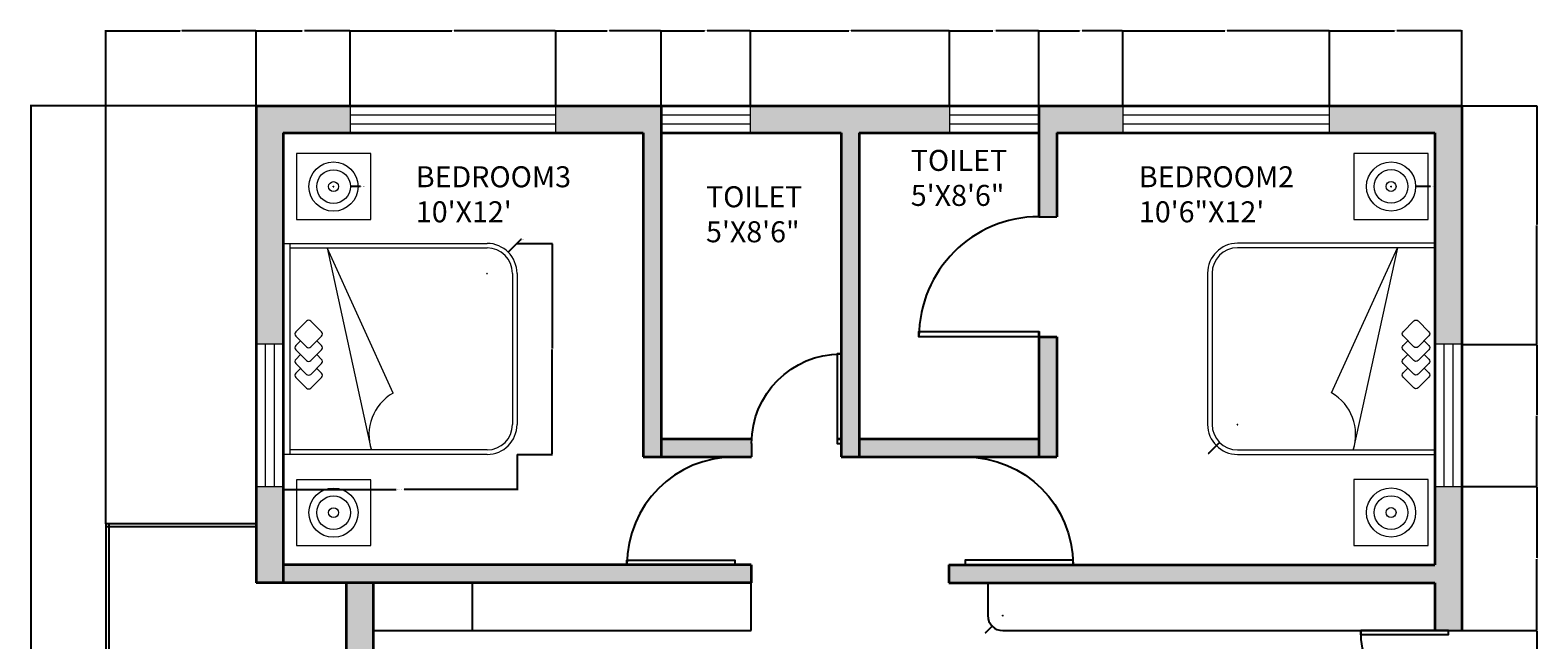
# Model space of a CAD drawing. Units: inches. Extents: x 2764 to 3282, y 1588 to 2106.
# Tile 2 of 2: x 2764 to 3267, y 1903 to 2106. Entities that reach past the tile are written whole.
import ezdxf

# ---------------------------------------------------------------- set-up
doc = ezdxf.new("R2010")
doc.units = ezdxf.units.IN
for name, color, linetype, lineweight in [('A-ANNO-DIMS', 2, 'Continuous', 18), ('A-AREA-IDEN', 7, 'Continuous', 25), ('A-DOOR', 3, 'Continuous', 25), ('A-FLOR-CASE', 8, 'Continuous', 25), ('A-FLOR-HRAL', 7, 'Continuous', 25), ('A-FURN', 8, 'Continuous', 18), ('A-GLAZ', 4, 'Continuous', 18), ('A-WALL', 7, 'Continuous', 35), ('A-WALL-PATT', 9, 'Continuous', 13)]:
    doc.layers.add(name, color=color, linetype=linetype, lineweight=lineweight)
doc.styles.get("Standard").update_dxf_attribs({"font": 'arial.ttf'})
doc.dimstyles.get("Standard").update_dxf_attribs({"dimtxt": 0.18, "dimasz": 0.18, "dimexe": 0.18, "dimexo": 0.0625, "dimgap": 0.09, "dimtad": 0, "dimtih": 1, "dimtoh": 1, "dimdec": 4, "dimzin": 0, "dimdsep": 46, "dimtxsty": 'Standard', "dimcen": 0.09, "dimadec": 0, "dimazin": 0, "dimtfac": 1, "dimtdec": 4, "dimtofl": 0, "dimtmove": 0, "dimatfit": 3, "dimfxl": 1, "dimtolj": 1, "dimtzin": 0, "dimarcsym": 0})

# ---------------------------------------------------------------- blocks, each defined once
blk = doc.blocks.new('*U2')
for p, q in [((0, 0), (0, -6)), ((40, 0), (40, -6))]:
    blk.add_line(p, q)
blk.add_lwpolyline([(0, 0), (0, 40), (1.75, 40), (1.75, 0)], close=True)
blk.add_arc((0, 0), 40, 0, 90)
blk = doc.blocks.new('SIDE-TABLE-WITH-LAMP')
for p, q in [((0, 21.93), (0, 0)), ((24.76, 21.93), (0, 21.93)), ((24.76, 0), (24.76, 21.93)), ((0, 0), (24.76, 0))]:
    blk.add_line(p, q)
for radius in [8.2, 5.62, 1.65]:
    blk.add_circle((12.38, 10.96), radius)
blk = doc.blocks.new('BED-DOUBLE')
for p, q in [((0, 70.34), (67.95, 70.34)), ((2.2, 70.34), (2.2, 0)), ((2.2, 68.84), (67.95, 68.84)), ((14.6, 68.84), (29.36, 1.5)), ((36.6, 20.47), (14.6, 68.84)), ((76.45, 60.34), (76.45, 10)), ((77.95, 60.34), (77.95, 10)), ((67.95, 0), (0, 0)), ((67.95, 1.5), (2.2, 1.5))]:
    blk.add_line(p, q)
blk.add_lwpolyline([(12.75, 40.88), (9.16, 44.46, 0.414214), (7.75, 44.46), (4.16, 40.88, 0.414214), (4.16, 39.46), (7.75, 35.88, 0.414214), (9.16, 35.88), (12.75, 39.46, 0.414214)], format="xyb", close=True)
for points in [[(5.75, 37.88), (4.16, 36.29, 0.414214), (4.16, 34.88), (7.75, 31.29, 0.414214), (9.16, 31.29), (12.75, 34.88, 0.414214), (12.75, 36.29), (11.16, 37.88)], [(5.75, 33.29), (4.16, 31.7, 0.414214), (4.16, 30.29), (7.75, 26.7, 0.414214), (9.16, 26.7), (12.75, 30.29, 0.414214), (12.75, 31.7), (11.16, 33.29)], [(5.75, 28.7), (4.16, 27.12, 0.414214), (4.16, 25.7), (7.75, 22.12, 0.414214), (9.16, 22.12), (12.75, 25.7, 0.414214), (12.75, 27.12), (11.16, 28.7)]]:
    blk.add_lwpolyline(points, format="xyb")
for centre, radius, start, end in [((67.95, 60.34), 10, 0, 90), ((67.95, 60.34), 8.5, 0, 90), ((44.61, 6.58), 16.03, 119.9541, 198.4829), ((67.95, 10), 10, 270, 0), ((67.95, 10), 8.5, 270, 0)]:
    blk.add_arc(centre, radius, start, end)
blk = doc.blocks.new('*D10')
at = {"layer": 'A-ANNO-DIMS', "color": 0, "lineweight": -2, "transparency": 16777216}
for p, q in [((2848.66, 1964.88), (2848.66, 1953.07)), ((2926.62, 1964.88), (2926.62, 1953.07)), ((2848.84, 1953.25), (2886.27, 1953.25)), ((2926.44, 1953.25), (2889.01, 1953.25))]:
    blk.add_line(p, q, dxfattribs=at)
at = {"layer": 'A-ANNO-DIMS', "color": 0, "transparency": 16777216}
for points in [[(2848.84, 1953.28), (2848.84, 1953.22), (2848.66, 1953.25)], [(2926.44, 1953.28), (2926.44, 1953.22), (2926.62, 1953.25)]]:
    blk.add_solid(points, dxfattribs=at)
at = {"layer": 'Defpoints', "color": 0, "transparency": 16777216}
for p in [(2848.66, 1964.94), (2926.62, 1964.94), (2926.62, 1953.25)]:
    blk.add_point(p, dxfattribs=at)
at = {"layer": 'A-ANNO-DIMS', "color": 0, "transparency": 16777216, "insert": (2887.64, 1953.25), "char_height": 0.18, "attachment_point": 5}
blk.add_mtext('\\A1;DOUBLE BED 78 TYP.', dxfattribs=at)
blk = doc.blocks.new('*D11')
at = {"layer": 'A-ANNO-DIMS', "color": 0, "lineweight": -2, "transparency": 16777216}
for p, q in [((2926.68, 2035.28), (2938.49, 2035.28)), ((2938.31, 2035.1), (2938.31, 2000.29)), ((2938.31, 1965.12), (2938.31, 1999.93)), ((2926.68, 1964.94), (2938.49, 1964.94))]:
    blk.add_line(p, q, dxfattribs=at)
at = {"layer": 'A-ANNO-DIMS', "color": 0, "transparency": 16777216}
for points in [[(2938.28, 2035.1), (2938.34, 2035.1), (2938.31, 2035.28)], [(2938.28, 1965.12), (2938.34, 1965.12), (2938.31, 1964.94)]]:
    blk.add_solid(points, dxfattribs=at)
at = {"layer": 'Defpoints', "color": 0, "transparency": 16777216}
for p in [(2926.62, 2035.28), (2938.31, 2035.28), (2926.62, 1964.94)]:
    blk.add_point(p, dxfattribs=at)
at = {"layer": 'A-ANNO-DIMS', "color": 0, "transparency": 16777216, "insert": (2938.31, 2000.11), "char_height": 0.18, "attachment_point": 5}
blk.add_mtext('\\A1;70 TYP.', dxfattribs=at)
blk = doc.blocks.new('*D19')
at = {"layer": 'A-ANNO-DIMS', "color": 0, "lineweight": -2, "transparency": 16777216}
for p, q in [((2839.6, 2081.14), (2764.28, 2081.14)), ((2764.46, 2080.96), (2764.46, 1847.33)), ((2764.46, 1613.32), (2764.46, 1846.96)), ((2839.6, 1613.14), (2764.28, 1613.14))]:
    blk.add_line(p, q, dxfattribs=at)
at = {"layer": 'A-ANNO-DIMS', "color": 0, "transparency": 16777216}
for points in [[(2764.43, 2080.96), (2764.49, 2080.96), (2764.46, 2081.14)], [(2764.43, 1613.32), (2764.49, 1613.32), (2764.46, 1613.14)]]:
    blk.add_solid(points, dxfattribs=at)
at = {"layer": 'Defpoints', "color": 0, "transparency": 16777216}
for p in [(2764.46, 2081.14), (2839.66, 2081.14), (2839.66, 1613.14)]:
    blk.add_point(p, dxfattribs=at)
at = {"layer": 'A-ANNO-DIMS', "color": 0, "transparency": 16777216, "insert": (2764.46, 1847.14), "char_height": 0.18, "attachment_point": 5}
blk.add_mtext('\\A1;468', dxfattribs=at)
blk = doc.blocks.new('*D20')
at = {"layer": 'A-ANNO-DIMS', "color": 0, "lineweight": -2, "transparency": 16777216}
for p, q in [((2789.46, 1941.87), (2789.46, 2106.32)), ((2789.64, 2106.14), (2814.24, 2106.14)), ((2839.48, 2106.14), (2814.88, 2106.14)), ((2839.66, 2081.21), (2839.66, 2106.32))]:
    blk.add_line(p, q, dxfattribs=at)
at = {"layer": 'A-ANNO-DIMS', "color": 0, "transparency": 16777216}
for points in [[(2789.64, 2106.17), (2789.64, 2106.11), (2789.46, 2106.14)], [(2839.48, 2106.17), (2839.48, 2106.11), (2839.66, 2106.14)]]:
    blk.add_solid(points, dxfattribs=at)
at = {"layer": 'Defpoints', "color": 0, "transparency": 16777216}
for p in [(2839.66, 2106.14), (2839.66, 2081.14), (2789.46, 1941.8)]:
    blk.add_point(p, dxfattribs=at)
at = {"layer": 'A-ANNO-DIMS', "color": 0, "transparency": 16777216, "insert": (2814.56, 2106.14), "char_height": 0.18, "attachment_point": 5}
blk.add_mtext('\\A1;50.2', dxfattribs=at)
blk = doc.blocks.new('*D21')
at = {"layer": 'A-ANNO-DIMS', "color": 0, "lineweight": -2, "transparency": 16777216}
for p, q in [((2839.66, 2081.21), (2839.66, 2106.32)), ((2839.84, 2106.14), (2854.94, 2106.14)), ((2870.83, 2106.14), (2855.73, 2106.14)), ((2871.01, 2081.21), (2871.01, 2106.32))]:
    blk.add_line(p, q, dxfattribs=at)
at = {"layer": 'A-ANNO-DIMS', "color": 0, "transparency": 16777216}
for points in [[(2839.84, 2106.17), (2839.84, 2106.11), (2839.66, 2106.14)], [(2870.83, 2106.17), (2870.83, 2106.11), (2871.01, 2106.14)]]:
    blk.add_solid(points, dxfattribs=at)
at = {"layer": 'Defpoints', "color": 0, "transparency": 16777216}
for p in [(2871.01, 2106.14), (2839.66, 2081.14), (2871.01, 2081.14)]:
    blk.add_point(p, dxfattribs=at)
at = {"layer": 'A-ANNO-DIMS', "color": 0, "transparency": 16777216, "insert": (2855.33, 2106.14), "char_height": 0.18, "attachment_point": 5}
blk.add_mtext('\\A1;31.35', dxfattribs=at)
blk = doc.blocks.new('*D22')
at = {"layer": 'A-ANNO-DIMS', "color": 0, "lineweight": -2, "transparency": 16777216}
for p, q in [((2871.01, 2081.21), (2871.01, 2106.32)), ((2871.19, 2106.14), (2904.88, 2106.14)), ((2939.36, 2106.14), (2905.67, 2106.14)), ((2939.54, 2081.21), (2939.54, 2106.32))]:
    blk.add_line(p, q, dxfattribs=at)
at = {"layer": 'A-ANNO-DIMS', "color": 0, "transparency": 16777216}
for points in [[(2871.19, 2106.17), (2871.19, 2106.11), (2871.01, 2106.14)], [(2939.36, 2106.17), (2939.36, 2106.11), (2939.54, 2106.14)]]:
    blk.add_solid(points, dxfattribs=at)
at = {"layer": 'Defpoints', "color": 0, "transparency": 16777216}
for p in [(2939.54, 2106.14), (2871.01, 2081.14), (2939.54, 2081.14)]:
    blk.add_point(p, dxfattribs=at)
at = {"layer": 'A-ANNO-DIMS', "color": 0, "transparency": 16777216, "insert": (2905.28, 2106.14), "char_height": 0.18, "attachment_point": 5}
blk.add_mtext('\\A1;68.53', dxfattribs=at)
blk = doc.blocks.new('*D23')
at = {"layer": 'A-ANNO-DIMS', "color": 0, "lineweight": -2, "transparency": 16777216}
for p, q in [((2939.54, 2081.21), (2939.54, 2106.32)), ((2939.72, 2106.14), (2956.71, 2106.14)), ((2974.48, 2106.14), (2957.49, 2106.14)), ((2974.66, 2081.21), (2974.66, 2106.32))]:
    blk.add_line(p, q, dxfattribs=at)
at = {"layer": 'A-ANNO-DIMS', "color": 0, "transparency": 16777216}
for points in [[(2939.72, 2106.17), (2939.72, 2106.11), (2939.54, 2106.14)], [(2974.48, 2106.17), (2974.48, 2106.11), (2974.66, 2106.14)]]:
    blk.add_solid(points, dxfattribs=at)
at = {"layer": 'Defpoints', "color": 0, "transparency": 16777216}
for p in [(2974.66, 2106.14), (2939.54, 2081.14), (2974.66, 2081.14)]:
    blk.add_point(p, dxfattribs=at)
at = {"layer": 'A-ANNO-DIMS', "color": 0, "transparency": 16777216, "insert": (2957.1, 2106.14), "char_height": 0.18, "attachment_point": 5}
blk.add_mtext('\\A1;35.12', dxfattribs=at)
blk = doc.blocks.new('*D24')
at = {"layer": 'A-ANNO-DIMS', "color": 0, "lineweight": -2, "transparency": 16777216}
for p, q in [((2974.66, 2081.21), (2974.66, 2106.32)), ((2974.84, 2106.14), (2989.08, 2106.14)), ((3004.25, 2106.14), (2990.01, 2106.14)), ((3004.43, 2081.21), (3004.43, 2106.32))]:
    blk.add_line(p, q, dxfattribs=at)
at = {"layer": 'A-ANNO-DIMS', "color": 0, "transparency": 16777216}
for points in [[(2974.84, 2106.17), (2974.84, 2106.11), (2974.66, 2106.14)], [(3004.25, 2106.17), (3004.25, 2106.11), (3004.43, 2106.14)]]:
    blk.add_solid(points, dxfattribs=at)
at = {"layer": 'Defpoints', "color": 0, "transparency": 16777216}
for p in [(3004.43, 2106.14), (2974.66, 2081.14), (3004.43, 2081.14)]:
    blk.add_point(p, dxfattribs=at)
at = {"layer": 'A-ANNO-DIMS', "color": 0, "transparency": 16777216, "insert": (2989.55, 2106.14), "char_height": 0.18, "attachment_point": 5}
blk.add_mtext('\\A1;29.774', dxfattribs=at)
blk = doc.blocks.new('*D25')
at = {"layer": 'A-ANNO-DIMS', "color": 0, "lineweight": -2, "transparency": 16777216}
for p, q in [((3004.43, 2081.21), (3004.43, 2106.32)), ((3004.61, 2106.14), (3037.27, 2106.14)), ((3070.71, 2106.14), (3038.06, 2106.14)), ((3070.89, 2081.21), (3070.89, 2106.32))]:
    blk.add_line(p, q, dxfattribs=at)
at = {"layer": 'A-ANNO-DIMS', "color": 0, "transparency": 16777216}
for points in [[(3004.61, 2106.17), (3004.61, 2106.11), (3004.43, 2106.14)], [(3070.71, 2106.17), (3070.71, 2106.11), (3070.89, 2106.14)]]:
    blk.add_solid(points, dxfattribs=at)
at = {"layer": 'Defpoints', "color": 0, "transparency": 16777216}
for p in [(3070.89, 2106.14), (3004.43, 2081.14), (3070.89, 2081.14)]:
    blk.add_point(p, dxfattribs=at)
at = {"layer": 'A-ANNO-DIMS', "color": 0, "transparency": 16777216, "insert": (3037.66, 2106.14), "char_height": 0.18, "attachment_point": 5}
blk.add_mtext('\\A1;66.45', dxfattribs=at)
blk = doc.blocks.new('*D26')
at = {"layer": 'A-ANNO-DIMS', "color": 0, "lineweight": -2, "transparency": 16777216}
for p, q in [((3070.89, 2081.21), (3070.89, 2106.32)), ((3071.07, 2106.14), (3085.31, 2106.14)), ((3100.48, 2106.14), (3086.24, 2106.14)), ((3100.66, 2081.21), (3100.66, 2106.32))]:
    blk.add_line(p, q, dxfattribs=at)
at = {"layer": 'A-ANNO-DIMS', "color": 0, "transparency": 16777216}
for points in [[(3071.07, 2106.17), (3071.07, 2106.11), (3070.89, 2106.14)], [(3100.48, 2106.17), (3100.48, 2106.11), (3100.66, 2106.14)]]:
    blk.add_solid(points, dxfattribs=at)
at = {"layer": 'Defpoints', "color": 0, "transparency": 16777216}
for p in [(3100.66, 2106.14), (3070.89, 2081.14), (3100.66, 2081.14)]:
    blk.add_point(p, dxfattribs=at)
at = {"layer": 'A-ANNO-DIMS', "color": 0, "transparency": 16777216, "insert": (3085.77, 2106.14), "char_height": 0.18, "attachment_point": 5}
blk.add_mtext('\\A1;29.774', dxfattribs=at)
blk = doc.blocks.new('*D27')
at = {"layer": 'A-ANNO-DIMS', "color": 0, "lineweight": -2, "transparency": 16777216}
for p, q in [((3100.66, 2081.21), (3100.66, 2106.32)), ((3100.84, 2106.14), (3114.16, 2106.14)), ((3128.42, 2106.14), (3115.09, 2106.14)), ((3128.6, 2081.21), (3128.6, 2106.32))]:
    blk.add_line(p, q, dxfattribs=at)
at = {"layer": 'A-ANNO-DIMS', "color": 0, "transparency": 16777216}
for points in [[(3100.84, 2106.17), (3100.84, 2106.11), (3100.66, 2106.14)], [(3128.42, 2106.17), (3128.42, 2106.11), (3128.6, 2106.14)]]:
    blk.add_solid(points, dxfattribs=at)
at = {"layer": 'Defpoints', "color": 0, "transparency": 16777216}
for p in [(3128.6, 2106.14), (3100.66, 2081.14), (3128.6, 2081.14)]:
    blk.add_point(p, dxfattribs=at)
at = {"layer": 'A-ANNO-DIMS', "color": 0, "transparency": 16777216, "insert": (3114.63, 2106.14), "char_height": 0.18, "attachment_point": 5}
blk.add_mtext('\\A1;27.937', dxfattribs=at)
blk = doc.blocks.new('*D28')
at = {"layer": 'A-ANNO-DIMS', "color": 0, "lineweight": -2, "transparency": 16777216}
for p, q in [((3128.6, 2081.21), (3128.6, 2106.32)), ((3128.78, 2106.14), (3162.69, 2106.14)), ((3197.4, 2106.14), (3163.48, 2106.14)), ((3197.58, 2081.21), (3197.58, 2106.32))]:
    blk.add_line(p, q, dxfattribs=at)
at = {"layer": 'A-ANNO-DIMS', "color": 0, "transparency": 16777216}
for points in [[(3128.78, 2106.17), (3128.78, 2106.11), (3128.6, 2106.14)], [(3197.4, 2106.17), (3197.4, 2106.11), (3197.58, 2106.14)]]:
    blk.add_solid(points, dxfattribs=at)
at = {"layer": 'Defpoints', "color": 0, "transparency": 16777216}
for p in [(3197.58, 2106.14), (3128.6, 2081.14), (3197.58, 2081.14)]:
    blk.add_point(p, dxfattribs=at)
at = {"layer": 'A-ANNO-DIMS', "color": 0, "transparency": 16777216, "insert": (3163.09, 2106.14), "char_height": 0.18, "attachment_point": 5}
blk.add_mtext('\\A1;68.98', dxfattribs=at)
blk = doc.blocks.new('*D29')
at = {"layer": 'A-ANNO-DIMS', "color": 0, "lineweight": -2, "transparency": 16777216}
for p, q in [((3197.58, 2081.21), (3197.58, 2106.32)), ((3197.76, 2106.14), (3219.22, 2106.14)), ((3241.48, 2106.14), (3220.02, 2106.14)), ((3241.66, 2081.21), (3241.66, 2106.32))]:
    blk.add_line(p, q, dxfattribs=at)
at = {"layer": 'A-ANNO-DIMS', "color": 0, "transparency": 16777216}
for points in [[(3197.76, 2106.17), (3197.76, 2106.11), (3197.58, 2106.14)], [(3241.48, 2106.17), (3241.48, 2106.11), (3241.66, 2106.14)]]:
    blk.add_solid(points, dxfattribs=at)
at = {"layer": 'Defpoints', "color": 0, "transparency": 16777216}
for p in [(3241.66, 2106.14), (3197.58, 2081.14), (3241.66, 2081.14)]:
    blk.add_point(p, dxfattribs=at)
at = {"layer": 'A-ANNO-DIMS', "color": 0, "transparency": 16777216, "insert": (3219.62, 2106.14), "char_height": 0.18, "attachment_point": 5}
blk.add_mtext('\\A1;44.08', dxfattribs=at)
blk = doc.blocks.new('*D34')
at = {"layer": 'A-ANNO-DIMS', "color": 0, "lineweight": -2, "transparency": 16777216}
for p, q in [((3241.72, 1906.27), (3266.84, 1906.27)), ((3266.66, 1906.09), (3266.66, 1891.82)), ((3266.66, 1877.19), (3266.66, 1891.46)), ((3241.72, 1877.01), (3266.84, 1877.01))]:
    blk.add_line(p, q, dxfattribs=at)
at = {"layer": 'A-ANNO-DIMS', "color": 0, "transparency": 16777216}
for points in [[(3266.63, 1906.09), (3266.69, 1906.09), (3266.66, 1906.27)], [(3266.63, 1877.19), (3266.69, 1877.19), (3266.66, 1877.01)]]:
    blk.add_solid(points, dxfattribs=at)
at = {"layer": 'Defpoints', "color": 0, "transparency": 16777216}
for p in [(3241.66, 1906.27), (3266.66, 1906.27), (3241.66, 1877.01)]:
    blk.add_point(p, dxfattribs=at)
at = {"layer": 'A-ANNO-DIMS', "color": 0, "transparency": 16777216, "insert": (3266.66, 1891.64), "char_height": 0.18, "attachment_point": 5}
blk.add_mtext('\\A1;29.253', dxfattribs=at)
blk = doc.blocks.new('*D35')
at = {"layer": 'A-ANNO-DIMS', "color": 0, "lineweight": -2, "transparency": 16777216}
for p, q in [((3241.72, 1954.3), (3266.84, 1954.3)), ((3266.66, 1954.12), (3266.66, 1930.46)), ((3266.66, 1906.45), (3266.66, 1930.1)), ((3241.72, 1906.27), (3266.84, 1906.27))]:
    blk.add_line(p, q, dxfattribs=at)
at = {"layer": 'A-ANNO-DIMS', "color": 0, "transparency": 16777216}
for points in [[(3266.63, 1954.12), (3266.69, 1954.12), (3266.66, 1954.3)], [(3266.63, 1906.45), (3266.69, 1906.45), (3266.66, 1906.27)]]:
    blk.add_solid(points, dxfattribs=at)
at = {"layer": 'Defpoints', "color": 0, "transparency": 16777216}
for p in [(3241.66, 1954.3), (3266.66, 1954.3), (3241.66, 1906.27)]:
    blk.add_point(p, dxfattribs=at)
at = {"layer": 'A-ANNO-DIMS', "color": 0, "transparency": 16777216, "insert": (3266.66, 1930.28), "char_height": 0.18, "attachment_point": 5}
blk.add_mtext('\\A1;48.03', dxfattribs=at)
blk = doc.blocks.new('*D36')
at = {"layer": 'A-ANNO-DIMS', "color": 0, "lineweight": -2, "transparency": 16777216}
for p, q in [((3241.72, 2001.64), (3266.84, 2001.64)), ((3266.66, 2001.46), (3266.66, 1978.15)), ((3266.66, 1954.48), (3266.66, 1977.79)), ((3241.72, 1954.3), (3266.84, 1954.3))]:
    blk.add_line(p, q, dxfattribs=at)
at = {"layer": 'A-ANNO-DIMS', "color": 0, "transparency": 16777216}
for points in [[(3266.63, 2001.46), (3266.69, 2001.46), (3266.66, 2001.64)], [(3266.63, 1954.48), (3266.69, 1954.48), (3266.66, 1954.3)]]:
    blk.add_solid(points, dxfattribs=at)
at = {"layer": 'Defpoints', "color": 0, "transparency": 16777216}
for p in [(3241.66, 2001.64), (3266.66, 2001.64), (3241.66, 1954.3)]:
    blk.add_point(p, dxfattribs=at)
at = {"layer": 'A-ANNO-DIMS', "color": 0, "transparency": 16777216, "insert": (3266.66, 1977.97), "char_height": 0.18, "attachment_point": 5}
blk.add_mtext('\\A1;47.35', dxfattribs=at)
blk = doc.blocks.new('*D37')
at = {"layer": 'A-ANNO-DIMS', "color": 0, "lineweight": -2, "transparency": 16777216}
for p, q in [((3241.72, 2081.14), (3266.84, 2081.14)), ((3266.66, 2080.96), (3266.66, 2041.58)), ((3266.66, 2001.82), (3266.66, 2041.21)), ((3241.72, 2001.64), (3266.84, 2001.64))]:
    blk.add_line(p, q, dxfattribs=at)
at = {"layer": 'A-ANNO-DIMS', "color": 0, "transparency": 16777216}
for points in [[(3266.63, 2080.96), (3266.69, 2080.96), (3266.66, 2081.14)], [(3266.63, 2001.82), (3266.69, 2001.82), (3266.66, 2001.64)]]:
    blk.add_solid(points, dxfattribs=at)
at = {"layer": 'Defpoints', "color": 0, "transparency": 16777216}
for p in [(3241.66, 2081.14), (3266.66, 2081.14), (3241.66, 2001.64)]:
    blk.add_point(p, dxfattribs=at)
at = {"layer": 'A-ANNO-DIMS', "color": 0, "transparency": 16777216, "insert": (3266.66, 2041.39), "char_height": 0.18, "attachment_point": 5}
blk.add_mtext('\\A1;79.5', dxfattribs=at)
blk = doc.blocks.new('*D39')
at = {"layer": 'A-ANNO-DIMS', "color": 0, "lineweight": -2, "transparency": 16777216}
for p, q in [((2927.93, 2036.59), (2923.81, 2032.48)), ((2928.11, 2036.59), (2927.93, 2036.59)), ((2916.53, 2025.28), (2916.71, 2025.28)), ((2916.62, 2025.19), (2916.62, 2025.37))]:
    blk.add_line(p, q, dxfattribs=at)
at = {"layer": 'A-ANNO-DIMS', "color": 0, "transparency": 16777216}
blk.add_solid([(2923.79, 2032.5), (2923.83, 2032.46), (2923.69, 2032.35)], dxfattribs=at)
at = {"layer": 'Defpoints', "color": 0, "transparency": 16777216}
for p in [(2923.69, 2032.35), (2916.62, 2025.28)]:
    blk.add_point(p, dxfattribs=at)
at = {"layer": 'A-ANNO-DIMS', "color": 0, "transparency": 16777216, "insert": (2928.61, 2036.59), "char_height": 0.18, "attachment_point": 5}
blk.add_mtext('\\A1;6X R10', dxfattribs=at)
blk = doc.blocks.new('*D40')
at = {"layer": 'A-ANNO-DIMS', "color": 0, "lineweight": -2, "transparency": 16777216}
for p, q in [((3166.81, 1974.98), (3166.99, 1974.98)), ((3166.9, 1974.89), (3166.9, 1975.07)), ((3157.29, 1965.36), (3160.77, 1968.84)), ((3157.11, 1965.36), (3157.29, 1965.36))]:
    blk.add_line(p, q, dxfattribs=at)
at = {"layer": 'A-ANNO-DIMS', "color": 0, "transparency": 16777216}
blk.add_solid([(3160.74, 1968.86), (3160.79, 1968.82), (3160.89, 1968.97)], dxfattribs=at)
at = {"layer": 'Defpoints', "color": 0, "transparency": 16777216}
for p in [(3166.9, 1974.98), (3160.89, 1968.97)]:
    blk.add_point(p, dxfattribs=at)
at = {"layer": 'A-ANNO-DIMS', "color": 0, "transparency": 16777216, "insert": (3156.57, 1965.36), "char_height": 0.18, "attachment_point": 5}
blk.add_mtext('\\A1;6X R8.5', dxfattribs=at)
blk = doc.blocks.new('*D41')
at = {"layer": 'A-ANNO-DIMS', "color": 0, "lineweight": -2, "transparency": 16777216}
for p, q in [((3218, 2054.25), (3218.18, 2054.25)), ((3218.09, 2054.16), (3218.09, 2054.34)), ((3231.21, 2054.25), (3226.47, 2054.25))]:
    blk.add_line(p, q, dxfattribs=at)
at = {"layer": 'A-ANNO-DIMS', "color": 0, "transparency": 16777216}
blk.add_solid([(3226.47, 2054.28), (3226.47, 2054.22), (3226.29, 2054.25)], dxfattribs=at)
at = {"layer": 'Defpoints', "color": 0, "transparency": 16777216}
for p in [(3209.88, 2054.25), (3226.29, 2054.25)]:
    blk.add_point(p, dxfattribs=at)
at = {"layer": 'A-ANNO-DIMS', "color": 0, "transparency": 16777216, "insert": (3231.94, 2054.25), "char_height": 0.18, "attachment_point": 5}
blk.add_mtext('\\A1;10X ∅16.41', dxfattribs=at)
blk = doc.blocks.new('*D42')
at = {"layer": 'A-ANNO-DIMS', "color": 0, "lineweight": -2, "transparency": 16777216}
for p, q in [((2865.34, 2054.21), (2865.52, 2054.21)), ((2865.43, 2054.12), (2865.43, 2054.3)), ((2874.43, 2054.21), (2871.24, 2054.21))]:
    blk.add_line(p, q, dxfattribs=at)
at = {"layer": 'A-ANNO-DIMS', "color": 0, "transparency": 16777216}
blk.add_solid([(2871.24, 2054.24), (2871.24, 2054.18), (2871.06, 2054.21)], dxfattribs=at)
at = {"layer": 'Defpoints', "color": 0, "transparency": 16777216}
for p in [(2859.81, 2054.21), (2871.06, 2054.21)]:
    blk.add_point(p, dxfattribs=at)
at = {"layer": 'A-ANNO-DIMS', "color": 0, "transparency": 16777216, "insert": (2875.17, 2054.21), "char_height": 0.18, "attachment_point": 5}
blk.add_mtext('\\A1;10X ∅11.25', dxfattribs=at)
blk = doc.blocks.new('*D46')
at = {"layer": 'A-ANNO-DIMS', "color": 0, "lineweight": -2, "transparency": 16777216}
for p, q in [((3088.51, 1911.27), (3088.69, 1911.27)), ((3088.6, 1911.18), (3088.6, 1911.36)), ((3082.77, 1905.61), (3082.95, 1905.61)), ((3082.95, 1905.61), (3084.94, 1907.6))]:
    blk.add_line(p, q, dxfattribs=at)
at = {"layer": 'A-ANNO-DIMS', "color": 0, "transparency": 16777216}
blk.add_solid([(3084.92, 1907.62), (3084.96, 1907.58), (3085.07, 1907.73)], dxfattribs=at)
at = {"layer": 'Defpoints', "color": 0, "transparency": 16777216}
for p in [(3088.6, 1911.27), (3085.07, 1907.73)]:
    blk.add_point(p, dxfattribs=at)
at = {"layer": 'A-ANNO-DIMS', "color": 0, "transparency": 16777216, "insert": (3082.53, 1905.61), "char_height": 0.18, "attachment_point": 5}
blk.add_mtext('\\A1;R5', dxfattribs=at)

msp = doc.modelspace()

# ---------------------------------------------------------------- hatches: boundary and pattern name
at = {"layer": 'A-WALL-PATT'}
h = msp.add_hatch(color=256, dxfattribs=at)
h.dxf.hatch_style = 1
h.paths.add_polyline_path([(2848.6606, 2072.1439), (2871.0084, 2072.1439), (2871.0084, 2081.1439), (2839.6606, 2081.1439), (2839.6606, 2001.6439), (2848.6606, 2001.6439)])
h.paths.add_polyline_path([(2974.6606, 2081.1439), (2939.543, 2081.1439), (2939.543, 2072.1439), (2968.6606, 2072.1439), (2968.6606, 1964.1439), (2974.6606, 1964.1439)])
h.paths.add_polyline_path([(3070.887, 2081.1439), (3004.4343, 2081.1439), (3004.4343, 2072.1439), (3034.6606, 2072.1439), (3034.6606, 1964.1439), (3040.6606, 1964.1439), (3040.6606, 2072.1439), (3070.887, 2072.1439)])
h.paths.add_polyline_path([(3128.5978, 2081.1439), (3100.6606, 2081.1439), (3100.6606, 2044.1785), (3106.6606, 2044.1785), (3106.6606, 2072.1439), (3128.5978, 2072.1439)])
h.paths.add_polyline_path([(3241.6606, 2081.1439), (3197.5781, 2081.1439), (3197.5781, 2072.1439), (3232.6606, 2072.1439), (3232.6606, 2001.6439), (3241.6606, 2001.6439)])
h.paths.add_polyline_path([(3106.6606, 2004.1785), (3100.6606, 2004.1785), (3100.6606, 1964.1439), (3106.6606, 1964.1439)])
h.paths.add_polyline_path([(3100.6606, 1970.1439), (3040.6606, 1970.1439), (3040.6606, 1964.1439), (3075.5248, 1964.1439, -0.00745077), (3076.5977, 1964.1439), (3100.6606, 1964.1439)])
h.paths.add_polyline_path([(3004.833, 1968.6181, -0.01279514), (3004.872, 1970.1439), (2974.6606, 1970.1439), (2974.6606, 1964.1439), (2998.0974, 1964.1439, -0.00805614), (2999.2578, 1964.1626), (3004.833, 1964.1626)])
h = msp.add_hatch(color=256, dxfattribs=at)
h.dxf.hatch_style = 1
h.paths.add_polyline_path([(2848.6606, 1954.2983), (2839.6606, 1954.2983), (2839.6606, 1922.1439), (2848.6606, 1922.1439)])
h.paths.add_polyline_path([(3004.6606, 1928.1439), (2999.2578, 1928.1439), (2963.2391, 1928.1439), (2848.6606, 1928.1439), (2848.6606, 1922.1439), (3004.6606, 1922.1439)])
h.paths.add_polyline_path([(3241.6606, 1954.2983), (3232.6606, 1954.2983), (3232.6606, 1928.1439), (3070.6606, 1928.1439), (3070.6606, 1922.1439), (3232.6606, 1922.1439), (3232.6606, 1906.2651), (3237.2727, 1906.2651), (3241.6606, 1906.2651)])
h.paths.add_polyline_path([(2878.6606, 1922.1439), (2869.6606, 1922.1439), (2869.6606, 1899.4014), (2878.6606, 1899.4014)])

# ---------------------------------------------------------------- linework, layer by layer
at = {"layer": 'A-FLOR-CASE'}
for p, q in [((2911.6562, 1922.1439), (2911.6562, 1906.2651)), ((3004.6606, 1906.2651), (3004.6606, 1922.1439)), ((3083.6041, 1922.1439), (3083.6041, 1911.2651)), ((2878.6606, 1906.2651), (3004.6606, 1906.2651)), ((3088.6041, 1906.2651), (3241.6606, 1906.2651))]:
    msp.add_line(p, q, dxfattribs=at)
msp.add_arc((3088.6041, 1911.2651), 5, 180, 270, dxfattribs=at)
at = {"layer": 'A-FLOR-HRAL'}
for p, q in [((2839.6606, 1941.8045), (2789.4608, 1941.8045)), ((2789.4608, 1941.8045), (2789.4608, 1752.7872)), ((2839.6606, 1940.8045), (2789.4608, 1940.8045)), ((2790.4608, 1941.8045), (2790.4608, 1752.7872))]:
    msp.add_line(p, q, dxfattribs=at)
at = {"layer": 'A-FURN'}
for p, q in [((3232.6606, 2035.3122), (3166.9033, 2035.3122)), ((3232.6606, 2033.8122), (3166.9033, 2033.8122)), ((3198.2534, 1985.4441), (3220.2567, 2033.8122)), ((3220.2567, 2033.8122), (3205.4924, 1966.4756)), ((3232.6606, 2035.3122), (3232.6606, 1964.9756)), ((3156.9033, 2025.3122), (3156.9033, 1974.9756)), ((3158.4033, 2025.3122), (3158.4033, 1974.9756)), ((3166.9033, 1966.4756), (3232.6606, 1966.4756)), ((3166.9033, 1964.9756), (3232.6606, 1964.9756))]:
    msp.add_line(p, q, dxfattribs=at)
msp.add_lwpolyline([(3222.109, 2005.851), (3225.6948, 2009.4368, -0.41421356), (3227.109, 2009.4368), (3230.6948, 2005.851, -0.41421356), (3230.6948, 2004.4368), (3227.109, 2000.851, -0.41421356), (3225.6948, 2000.851), (3222.109, 2004.4368, -0.41421356)], format="xyb", close=True, dxfattribs=at)
for points in [[(3229.109, 2002.851), (3230.6948, 2001.2653, -0.41421356), (3230.6948, 1999.851), (3227.109, 1996.2653, -0.41421356), (3225.6948, 1996.2653), (3222.109, 1999.851, -0.41421356), (3222.109, 2001.2653), (3223.6948, 2002.851)], [(3229.109, 1998.2653), (3230.6948, 1996.6795, -0.41421356), (3230.6948, 1995.2653), (3227.109, 1991.6795, -0.41421356), (3225.6948, 1991.6795), (3222.109, 1995.2653, -0.41421356), (3222.109, 1996.6795), (3223.6948, 1998.2653)], [(3229.109, 1993.6795), (3230.6948, 1992.0937, -0.41421356), (3230.6948, 1990.6795), (3227.109, 1987.0937, -0.41421356), (3225.6948, 1987.0937), (3222.109, 1990.6795, -0.41421356), (3222.109, 1992.0937), (3223.6948, 1993.6795)]]:
    msp.add_lwpolyline(points, format="xyb", dxfattribs=at)
for centre, radius, start, end in [((3166.9033, 2025.3122), 10, 90, 180), ((3166.9033, 2025.3122), 8.5, 90, 180), ((3190.2504, 1971.5569), 16.0281, 341.517131, 60.045889), ((3166.9033, 1974.9756), 10, 180, 270), ((3166.9033, 1974.9756), 8.5, 180, 270)]:
    msp.add_arc(centre, radius, start, end, dxfattribs=at)
at = {"layer": 'A-GLAZ'}
for p, q in [((2871.0084, 2081.1439), (2871.0084, 2072.1439)), ((2871.0084, 2078.1439), (2939.543, 2078.1439)), ((2939.543, 2072.1439), (2939.543, 2081.1439)), ((2974.6606, 2081.1439), (2974.6606, 2072.1439)), ((2974.6606, 2078.1439), (3004.4343, 2078.1439)), ((3004.4343, 2072.1439), (3004.4343, 2081.1439)), ((3100.6606, 2081.1439), (3070.887, 2081.1439)), ((3070.887, 2081.1439), (3070.887, 2072.1439)), ((3070.887, 2078.1439), (3100.6606, 2078.1439)), ((3128.5978, 2081.1439), (3128.5978, 2072.1439)), ((3197.5781, 2081.1439), (3128.5978, 2081.1439)), ((3128.5978, 2078.1439), (3197.5781, 2078.1439)), ((3197.5781, 2072.1439), (3197.5781, 2081.1439)), ((2871.0084, 2075.1439), (2939.543, 2075.1439)), ((2871.0084, 2072.1439), (2939.543, 2072.1439)), ((2974.6606, 2075.1439), (3004.4343, 2075.1439)), ((3070.887, 2075.1439), (3100.6606, 2075.1439)), ((3070.887, 2072.1439), (3100.6606, 2072.1439)), ((3128.5978, 2075.1439), (3197.5781, 2075.1439)), ((3128.5978, 2072.1439), (3197.5781, 2072.1439)), ((2848.6606, 2001.6439), (2839.6606, 2001.6439)), ((2842.6606, 2001.6439), (2842.6606, 1954.2983)), ((2845.6606, 2001.6439), (2845.6606, 1954.2983)), ((3241.6606, 2001.6439), (3232.6606, 2001.6439)), ((3232.6606, 2001.6439), (3232.6606, 1954.2983)), ((3235.6606, 2001.6439), (3235.6606, 1954.2983)), ((3238.6606, 2001.6439), (3238.6606, 1954.2983)), ((3241.6606, 1954.2983), (3241.6606, 2001.6439)), ((2839.6606, 1954.2983), (2848.6606, 1954.2983)), ((3232.6606, 1954.2983), (3241.6606, 1954.2983))]:
    msp.add_line(p, q, dxfattribs=at)
at = {"layer": 'A-WALL'}
for p, q in [((2839.6606, 2081.1439), (3241.6606, 2081.1439)), ((2839.6606, 2081.1439), (2839.6606, 1922.1439)), ((2974.6606, 2081.1439), (2974.6606, 1964.1439)), ((3100.6606, 2081.1439), (3100.6606, 2044.1785)), ((3241.6606, 2081.1439), (3241.6606, 1906.2651)), ((2848.6606, 2072.1439), (2968.6606, 2072.1439)), ((2848.6606, 2072.1439), (2848.6606, 1922.1439)), ((2968.6606, 2072.1439), (2968.6606, 1964.1439)), ((2974.6606, 2072.1439), (3034.6606, 2072.1439)), ((3034.6606, 2072.1439), (3034.6606, 1964.1439)), ((3040.6606, 2072.1439), (3040.6606, 1964.1439)), ((3040.6606, 2072.1439), (3100.6606, 2072.1439)), ((3106.6606, 2072.1439), (3106.6606, 2044.1785)), ((3106.6606, 2072.1439), (3232.6606, 2072.1439)), ((3232.6606, 2072.1439), (3232.6606, 1928.1439)), ((3100.6606, 2005.9285), (3100.6606, 1964.1439)), ((3100.6606, 2004.1785), (3106.6606, 2004.1785)), ((3106.6606, 2004.1785), (3106.6606, 1964.1439)), ((2974.6606, 1970.1439), (3004.872, 1970.1439)), ((3033.3557, 1970.1439), (3034.6606, 1970.1439)), ((3040.6606, 1970.1439), (3100.6606, 1970.1439)), ((2968.6606, 1964.1439), (3004.833, 1964.1439)), ((3034.6606, 1964.1439), (3040.6606, 1964.1439)), ((3040.6606, 1964.1439), (3106.6606, 1964.1439)), ((3004.6606, 1928.1439), (2848.6606, 1928.1439)), ((3004.6606, 1928.1439), (3004.6606, 1922.1439)), ((3070.6606, 1928.1439), (3232.6606, 1928.1439)), ((3070.6606, 1928.1439), (3070.6606, 1922.1439)), ((3004.6606, 1922.1439), (2839.6606, 1922.1439)), ((2869.6606, 1922.1439), (2869.6606, 1778.1439)), ((2878.6606, 1922.1439), (2878.6606, 1778.1439)), ((3070.6606, 1922.1439), (3232.6606, 1922.1439)), ((3232.6606, 1922.1439), (3232.6606, 1906.2651))]:
    msp.add_line(p, q, dxfattribs=at)

# ---------------------------------------------------------------- block references
at = {"layer": 'A-DOOR', "rotation": 89.99999999999999}
msp.add_blockref('*U2', (3100.6606, 2004.1785), dxfattribs=at)
at = {"layer": 'A-DOOR', "xscale": -0.7456920988934935, "yscale": 0.7456920988934935, "zscale": 0.7456920988934935}
msp.add_blockref('*U2', (3034.6606, 1968.6181), dxfattribs=at)
at = {"layer": 'A-DOOR'}
for p, xscale, yscale, zscale, rotation in [((2999.2578, 1928.1439), 0.9004674725941558, 0.9004674725941558, 0.9004674725941558, 89.99999999999999), ((3076.0612, 1928.1439), -0.9000999306307651, 0.9000999306307651, 0.9000999306307651, 270), ((3237.2727, 1906.2651), -0.731332392084942, 0.731332392084942, 0.731332392084942, 90)]:
    msp.add_blockref('*U2', p, dxfattribs=dict(at, xscale=xscale, yscale=yscale, zscale=zscale, rotation=rotation))
at = {"layer": 'A-FURN'}
for name, p in [('SIDE-TABLE-WITH-LAMP', (2853.05, 2043.248)), ('BED-DOUBLE', (2848.661, 1964.941)), ('SIDE-TABLE-WITH-LAMP', (2853.05, 1934.5941))]:
    msp.add_blockref(name, p, dxfattribs=at)
at = {"layer": 'A-FURN', "rotation": 180}
for p in [(3230.4683, 2065.2092), (3230.4683, 1956.5553)]:
    msp.add_blockref('SIDE-TABLE-WITH-LAMP', p, dxfattribs=at)

# ---------------------------------------------------------------- texts
at = {"layer": 'A-AREA-IDEN', "char_height": 7, "attachment_point": 1}
for s, insert in [('TOILET\\P5\'X8\'6"', (3057.9337, 2066.442)), ("BEDROOM3\\P10'X12'", (2892.8763, 2060.9726)), ('BEDROOM2\\P10\'6"X12\'', (3133.9958, 2060.9726)), ('TOILET\\P5\'X8\'6"', (2989.6386, 2054.3156))]:
    msp.add_mtext_dynamic_manual_height_columns(s, width=45.041222, gutter_width=12.5, heights=[0], dxfattribs=dict(at, insert=insert))

# ---------------------------------------------------------------- dimensions: what is measured, and where the dimension line sits
at = {"layer": 'A-ANNO-DIMS'}
for base, p1, p2, override, picture, middle in [((2839.6606, 2106.1439), (2789.4608, 1941.8045), (2839.6606, 2081.1439), {"dimdec": 1, "dimlfac": 1, "dimrnd": 0, "dimzin": 0, "dimdsep": 46, "dimlunit": 2}, '*D20', (2814.5607, 2106.1439)), ((2871.0084, 2106.1439), (2839.6606, 2081.1439), (2871.0084, 2081.1439), {"dimdec": 2, "dimlfac": 1, "dimrnd": 0, "dimzin": 0, "dimdsep": 46, "dimlunit": 2}, '*D21', (2855.3345, 2106.1439)), ((2939.543, 2106.1439), (2871.0084, 2081.1439), (2939.543, 2081.1439), {"dimdec": 2, "dimlfac": 1, "dimrnd": 0, "dimzin": 0, "dimdsep": 46, "dimlunit": 2}, '*D22', (2905.2757, 2106.1439)), ((2974.6606, 2106.1439), (2939.543, 2081.1439), (2974.6606, 2081.1439), {"dimdec": 2, "dimlfac": 1, "dimrnd": 0, "dimzin": 0, "dimdsep": 46, "dimlunit": 2}, '*D23', (2957.1018, 2106.1439)), ((3004.4343, 2106.1439), (2974.6606, 2081.1439), (3004.4343, 2081.1439), {"dimdec": 3, "dimlfac": 1, "dimrnd": 0, "dimzin": 0, "dimdsep": 46, "dimlunit": 2}, '*D24', (2989.5475, 2106.1439)), ((3070.887, 2106.1439), (3004.4343, 2081.1439), (3070.887, 2081.1439), {"dimdec": 2, "dimlfac": 1, "dimrnd": 0, "dimzin": 0, "dimdsep": 46, "dimlunit": 2}, '*D25', (3037.6606, 2106.1439)), ((3100.6606, 2106.1439), (3070.887, 2081.1439), (3100.6606, 2081.1439), {"dimdec": 3, "dimlfac": 1, "dimrnd": 0, "dimzin": 0, "dimdsep": 46, "dimlunit": 2}, '*D26', (3085.7738, 2106.1439)), ((3128.5978, 2106.1439), (3100.6606, 2081.1439), (3128.5978, 2081.1439), {"dimdec": 3, "dimlfac": 1, "dimrnd": 0, "dimzin": 0, "dimdsep": 46, "dimlunit": 2}, '*D27', (3114.6292, 2106.1439)), ((3197.5781, 2106.1439), (3128.5978, 2081.1439), (3197.5781, 2081.1439), {"dimdec": 2, "dimlfac": 1, "dimrnd": 0, "dimzin": 0, "dimdsep": 46, "dimlunit": 2}, '*D28', (3163.088, 2106.1439)), ((3241.6606, 2106.1439), (3197.5781, 2081.1439), (3241.6606, 2081.1439), {"dimdec": 2, "dimlfac": 1, "dimrnd": 0, "dimzin": 0, "dimdsep": 46, "dimlunit": 2}, '*D29', (3219.6194, 2106.1439))]:
    dim = msp.add_linear_dim(base=base, p1=p1, p2=p2, dimstyle='Standard', override=override, dxfattribs=at)
    dim.commit()
    dim.dimension.update_dxf_attribs({"geometry": picture, "text_midpoint": middle})
for base, p1, p2, override, picture, middle in [((2764.4608, 2081.1439), (2839.6606, 1613.1439), (2839.6606, 2081.1439), {"dimdec": 0, "dimlfac": 1, "dimrnd": 0, "dimzin": 0, "dimdsep": 46, "dimlunit": 2}, '*D19', (2764.4608, 1847.1439)), ((3266.6606, 2081.1439), (3241.6606, 2001.6439), (3241.6606, 2081.1439), {"dimdec": 1, "dimlfac": 1, "dimrnd": 0, "dimzin": 0, "dimdsep": 46, "dimlunit": 2}, '*D37', (3266.6606, 2041.3939)), ((3266.6606, 2001.6439), (3241.6606, 1954.2983), (3241.6606, 2001.6439), {"dimdec": 2, "dimlfac": 1, "dimrnd": 0, "dimzin": 0, "dimdsep": 46, "dimlunit": 2}, '*D36', (3266.6606, 1977.9711)), ((3266.6606, 1954.2983), (3241.6606, 1906.2651), (3241.6606, 1954.2983), {"dimdec": 2, "dimlfac": 1, "dimrnd": 0, "dimzin": 0, "dimdsep": 46, "dimlunit": 2}, '*D35', (3266.6606, 1930.2817)), ((3266.6606, 1906.2651), (3241.6606, 1877.0118), (3241.6606, 1906.2651), {"dimdec": 3, "dimlfac": 1, "dimrnd": 0, "dimzin": 0, "dimdsep": 46, "dimlunit": 2}, '*D34', (3266.6606, 1891.6385))]:
    dim = msp.add_linear_dim(base=base, p1=p1, p2=p2, angle=90, dimstyle='Standard', override=override, dxfattribs=at)
    dim.commit()
    dim.dimension.update_dxf_attribs({"geometry": picture, "text_midpoint": middle})
for p1, p2, picture, middle in [((2859.8062, 2054.2119), (2871.0556, 2054.211), '*D42', (2874.4304, 2054.2107)), ((3209.8828, 2054.2455), (3226.2921, 2054.246), '*D41', (3231.2148, 2054.2462))]:
    dim = msp.add_diameter_dim_2p(p1=p1, p2=p2, text='10X <>', dimstyle='Standard', override={"dimdec": 2, "dimlfac": 1, "dimrnd": 0, "dimzin": 0, "dimdsep": 46, "dimlunit": 2}, dxfattribs=at)
    dim.commit()
    dim.dimension.update_dxf_attribs({"geometry": picture, "text_midpoint": middle, "dimtype": 163})
for center, mpoint, override, picture, middle in [((2916.6151, 2025.2779), (2923.6861, 2032.3491), {"dimdec": 0, "dimlfac": 1, "dimrnd": 0, "dimzin": 0, "dimdsep": 46, "dimlunit": 2}, '*D39', (2928.6073, 2036.5917)), ((3166.9033, 1974.9756), (3160.893, 1968.965), {"dimdec": 1, "dimlfac": 1, "dimrnd": 0, "dimzin": 0, "dimdsep": 46, "dimlunit": 2}, '*D40', (3156.5724, 1965.3587))]:
    dim = msp.add_radius_dim(center=center, mpoint=mpoint, text='6X <>', dimstyle='Standard', override=override, dxfattribs=at)
    dim.commit()
    dim.dimension.update_dxf_attribs({"geometry": picture, "text_midpoint": middle, "dimtype": 164})
dim = msp.add_linear_dim(base=(2938.3082, 2035.2779), p1=(2926.6151, 1964.9413), p2=(2926.6151, 2035.2779), angle=90, text='<> TYP.', dimstyle='Standard', override={"dimdec": 0, "dimlfac": 1, "dimrnd": 0, "dimzin": 0, "dimdsep": 46, "dimlunit": 2}, dxfattribs=at)
dim.commit()
dim.dimension.update_dxf_attribs({"geometry": '*D11', "text_midpoint": (2938.3082, 2000.1096)})
dim = msp.add_linear_dim(base=(2926.6151, 1953.2482), p1=(2848.6606, 1964.9413), p2=(2926.6151, 1964.9413), text='DOUBLE BED <> TYP.', dimstyle='Standard', override={"dimdec": 0, "dimlfac": 1, "dimrnd": 0, "dimzin": 0, "dimdsep": 46, "dimlunit": 2}, dxfattribs=at)
dim.commit()
dim.dimension.update_dxf_attribs({"geometry": '*D10', "text_midpoint": (2887.6379, 1953.2482)})
dim = msp.add_radius_dim(center=(3088.6041, 1911.2651), mpoint=(3085.0686, 1907.7296), dimstyle='Standard', override={"dimdec": 0, "dimlfac": 1, "dimrnd": 0, "dimzin": 0, "dimdsep": 46, "dimlunit": 2}, dxfattribs=at)
dim.commit()
dim.dimension.update_dxf_attribs({"geometry": '*D46', "text_midpoint": (3082.5314, 1905.6083), "dimtype": 164})

doc.saveas('drawing.dxf')
